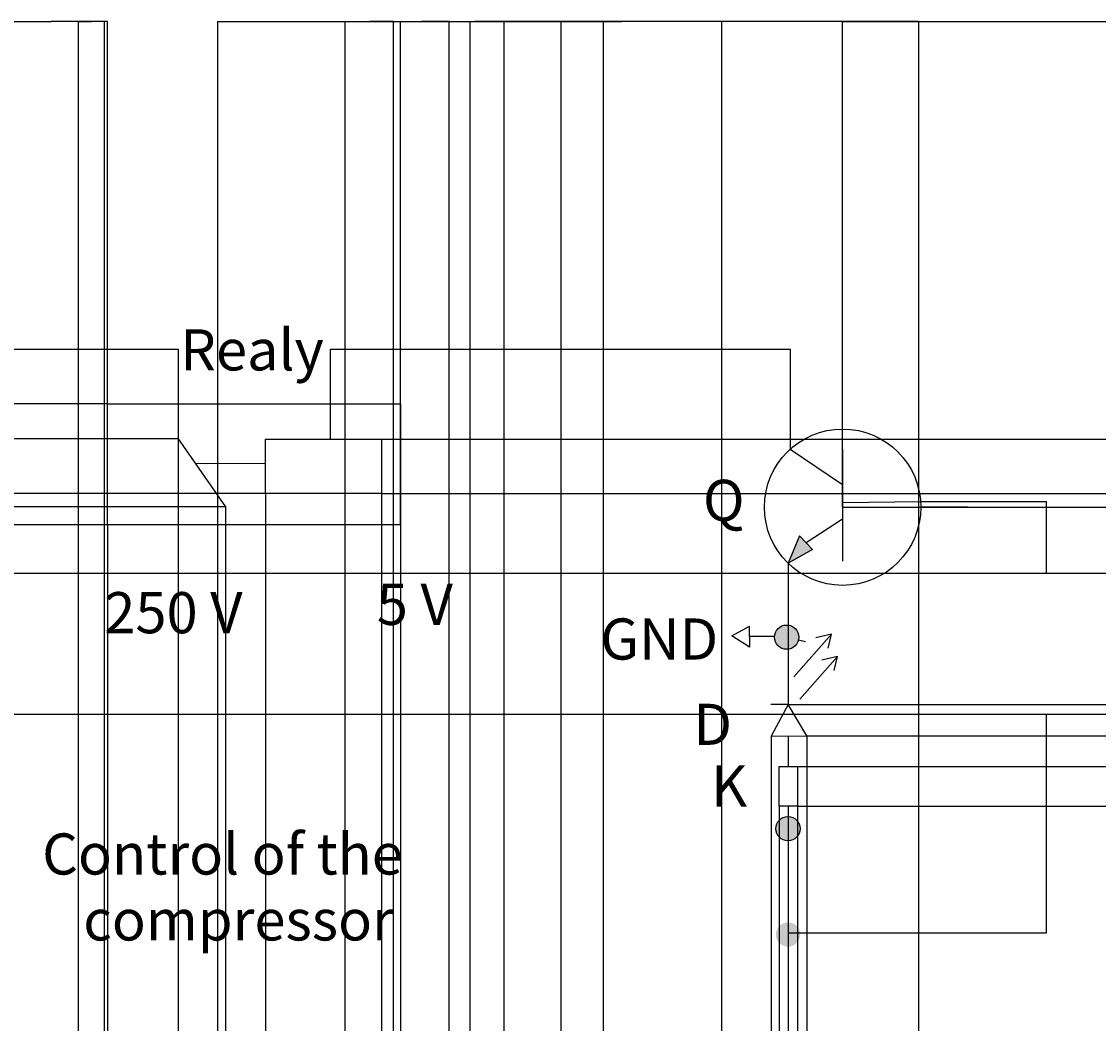
# Model space of a CAD drawing. Units: inches. Extents: x 35362 to 73946, y 43607 to 67532.
# Tile 132 of 134: x 52056 to 57838, y 62152 to 67532. Entities that reach past the tile are written whole.
import ezdxf

# ---------------------------------------------------------------- set-up
doc = ezdxf.new("R2010")
doc.units = ezdxf.units.IN
doc.header["$MEASUREMENT"] = 0
for name, color, linetype, lineweight in [('A-ANNO-DIMS', 2, 'Continuous', 18), ('E-ANNO-TEXT', 5, 'Continuous', 18), ('E-SYMB', 1, 'Continuous', 25), ('E-SYMB-PATT', 1, 'Continuous', 13), ('E-WIRE', 3, 'Continuous', 25)]:
    doc.layers.add(name, color=color, linetype=linetype, lineweight=lineweight)
doc.styles.get("Standard").update_dxf_attribs({"font": 'arial.ttf'})
doc.dimstyles.get("Standard").update_dxf_attribs({"dimtxt": 0.18, "dimasz": 0.18, "dimexe": 0.18, "dimexo": 0.0625, "dimgap": 0.09, "dimtad": 0, "dimtih": 1, "dimtoh": 1, "dimdec": 4, "dimzin": 0, "dimdsep": 46, "dimtxsty": 'Standard', "dimcen": 0.09, "dimadec": 0, "dimazin": 0, "dimtfac": 1, "dimtdec": 4, "dimtofl": 0, "dimtmove": 0, "dimatfit": 3, "dimfxl": 1, "dimtolj": 1, "dimtzin": 0, "dimarcsym": 0})

# ---------------------------------------------------------------- blocks, each defined once
blk = doc.blocks.new('*D9')
at = {"layer": 'A-ANNO-DIMS', "color": 0, "lineweight": -2, "transparency": 16777216}
for p, q in [((56873.6, 59185.2), (56873.6, 67531.7)), ((56873.8, 67531.5), (59056.9, 67531.5)), ((61240.7, 67531.5), (59057.6, 67531.5)), ((61240.9, 59185.2), (61240.9, 67531.7))]:
    blk.add_line(p, q, dxfattribs=at)
at = {"layer": 'A-ANNO-DIMS', "color": 0, "transparency": 16777216}
for points in [[(56873.8, 67531.5), (56873.8, 67531.5), (56873.6, 67531.5)], [(61240.7, 67531.5), (61240.7, 67531.5), (61240.9, 67531.5)]]:
    blk.add_solid(points, dxfattribs=at)
at = {"layer": 'Defpoints', "color": 0, "transparency": 16777216}
for p in [(61240.9, 67531.5), (56873.6, 59185.1), (61240.9, 59185.1)]:
    blk.add_point(p, dxfattribs=at)
at = {"layer": 'A-ANNO-DIMS', "color": 0, "transparency": 16777216, "insert": (59057.3, 67531.5), "char_height": 0.18, "attachment_point": 5}
blk.add_mtext('\\A1;4367', dxfattribs=at)
blk = doc.blocks.new('*D20')
at = {"layer": 'A-ANNO-DIMS', "color": 0, "lineweight": -2, "transparency": 16777216}
for p, q in [((56464.6, 64923.8), (56464.8, 64923.8)), ((56464.7, 64923.7), (56464.7, 64923.8)), ((57136.4, 64924), (56884.7, 64923.9))]:
    blk.add_line(p, q, dxfattribs=at)
at = {"layer": 'A-ANNO-DIMS', "color": 0, "transparency": 16777216}
blk.add_solid([(56884.7, 64923.9), (56884.7, 64923.8), (56884.5, 64923.9)], dxfattribs=at)
at = {"layer": 'Defpoints', "color": 0, "transparency": 16777216}
for p in [(56044.9, 64923.6), (56884.5, 64923.9)]:
    blk.add_point(p, dxfattribs=at)
at = {"layer": 'A-ANNO-DIMS', "color": 0, "transparency": 16777216, "insert": (57137.1, 64924), "char_height": 0.18, "attachment_point": 5}
blk.add_mtext('\\A1;2X ∅839.6', dxfattribs=at)
blk = doc.blocks.new('*D22')
at = {"layer": 'A-ANNO-DIMS', "color": 0, "lineweight": -2, "transparency": 16777216}
for p, q in [((56163.8, 64225.8), (56164, 64225.8)), ((56163.9, 64225.7), (56163.9, 64225.9)), ((56265.4, 64201.7), (56227.5, 64210.7))]:
    blk.add_line(p, q, dxfattribs=at)
at = {"layer": 'A-ANNO-DIMS', "color": 0, "transparency": 16777216}
blk.add_solid([(56227.5, 64210.7), (56227.5, 64210.7), (56227.3, 64210.7)], dxfattribs=at)
at = {"layer": 'Defpoints', "color": 0, "transparency": 16777216}
for p in [(56100.5, 64240.9), (56227.3, 64210.7)]:
    blk.add_point(p, dxfattribs=at)
at = {"layer": 'A-ANNO-DIMS', "color": 0, "transparency": 16777216, "insert": (56266.1, 64201.7), "char_height": 0.18, "attachment_point": 5}
blk.add_mtext('\\A1;4X ∅130.4', dxfattribs=at)
blk = doc.blocks.new('*D25')
at = {"layer": 'A-ANNO-DIMS', "color": 0, "lineweight": -2, "transparency": 16777216}
for p, q in [((53109.8, 59023.3), (53109.8, 67531.7)), ((53109.9, 67531.5), (54991.2, 67531.5)), ((56873.4, 67531.5), (54992.1, 67531.5)), ((56873.6, 59185.2), (56873.6, 67531.7))]:
    blk.add_line(p, q, dxfattribs=at)
at = {"layer": 'A-ANNO-DIMS', "color": 0, "transparency": 16777216}
for points in [[(53109.9, 67531.5), (53109.9, 67531.5), (53109.8, 67531.5)], [(56873.4, 67531.5), (56873.4, 67531.5), (56873.6, 67531.5)]]:
    blk.add_solid(points, dxfattribs=at)
at = {"layer": 'Defpoints', "color": 0, "transparency": 16777216}
for p in [(56873.6, 67531.5), (56873.6, 59185.1), (53109.8, 59023.3)]:
    blk.add_point(p, dxfattribs=at)
at = {"layer": 'A-ANNO-DIMS', "color": 0, "transparency": 16777216, "insert": (54991.7, 67531.5), "char_height": 0.18, "attachment_point": 5}
blk.add_mtext('\\A1;3763.8', dxfattribs=at)
blk = doc.blocks.new('*D29')
at = {"layer": 'A-ANNO-DIMS', "color": 0, "lineweight": -2, "transparency": 16777216}
for p, q in [((51913.9, 64127.5), (51913.9, 67531.7)), ((51914.1, 67531.5), (52215.5, 67531.5)), ((52517.6, 67531.5), (52216.3, 67531.5)), ((52517.8, 64828.6), (52517.8, 67531.7))]:
    blk.add_line(p, q, dxfattribs=at)
at = {"layer": 'A-ANNO-DIMS', "color": 0, "transparency": 16777216}
for points in [[(51914.1, 67531.5), (51914.1, 67531.5), (51913.9, 67531.5)], [(52517.6, 67531.5), (52517.6, 67531.5), (52517.8, 67531.5)]]:
    blk.add_solid(points, dxfattribs=at)
at = {"layer": 'Defpoints', "color": 0, "transparency": 16777216}
for p in [(52517.8, 67531.5), (52517.8, 64828.6), (51913.9, 64127.4)]:
    blk.add_point(p, dxfattribs=at)
at = {"layer": 'A-ANNO-DIMS', "color": 0, "transparency": 16777216, "insert": (52215.9, 67531.5), "char_height": 0.18, "attachment_point": 5}
blk.add_mtext('\\A1;603.9', dxfattribs=at)
blk = doc.blocks.new('*D30')
at = {"layer": 'A-ANNO-DIMS', "color": 0, "lineweight": -2, "transparency": 16777216}
for p, q in [((54090.8, 64828.6), (54090.8, 67531.7)), ((54090.9, 67531.5), (55277.3, 67531.5)), ((56464.6, 67531.5), (55278.2, 67531.5)), ((56464.7, 64923.8), (56464.7, 67531.7))]:
    blk.add_line(p, q, dxfattribs=at)
at = {"layer": 'A-ANNO-DIMS', "color": 0, "transparency": 16777216}
for points in [[(54090.9, 67531.5), (54090.9, 67531.5), (54090.8, 67531.5)], [(56464.6, 67531.5), (56464.6, 67531.5), (56464.7, 67531.5)]]:
    blk.add_solid(points, dxfattribs=at)
at = {"layer": 'Defpoints', "color": 0, "transparency": 16777216}
for p in [(56464.7, 67531.5), (56464.7, 64923.8), (54090.8, 64828.6)]:
    blk.add_point(p, dxfattribs=at)
at = {"layer": 'A-ANNO-DIMS', "color": 0, "transparency": 16777216, "insert": (55277.8, 67531.5), "char_height": 0.18, "attachment_point": 5}
blk.add_mtext('\\A1;2374.0', dxfattribs=at)
blk = doc.blocks.new('*D31')
at = {"layer": 'A-ANNO-DIMS', "color": 0, "lineweight": -2, "transparency": 16777216}
for p, q in [((56464.7, 64923.8), (56464.7, 67531.7)), ((56464.9, 67531.5), (58624.5, 67531.5)), ((60785, 67531.5), (58625.4, 67531.5)), ((60785.2, 64923.8), (60785.2, 67531.7))]:
    blk.add_line(p, q, dxfattribs=at)
at = {"layer": 'A-ANNO-DIMS', "color": 0, "transparency": 16777216}
for points in [[(56464.9, 67531.5), (56464.9, 67531.5), (56464.7, 67531.5)], [(60785, 67531.5), (60785, 67531.5), (60785.2, 67531.5)]]:
    blk.add_solid(points, dxfattribs=at)
at = {"layer": 'Defpoints', "color": 0, "transparency": 16777216}
for p in [(60785.2, 67531.5), (56464.7, 64923.8), (60785.2, 64923.8)]:
    blk.add_point(p, dxfattribs=at)
at = {"layer": 'A-ANNO-DIMS', "color": 0, "transparency": 16777216, "insert": (58625, 67531.5), "char_height": 0.18, "attachment_point": 5}
blk.add_mtext('\\A1;4320.5', dxfattribs=at)
blk = doc.blocks.new('*D39')
at = {"layer": 'A-ANNO-DIMS', "color": 0, "lineweight": -2, "transparency": 16777216}
for p, q in [((53793.6, 46128.9), (53793.6, 67531.7)), ((53793.8, 67531.5), (54487.2, 67531.5)), ((55181.5, 67531.5), (54488.1, 67531.5)), ((55181.6, 46128.9), (55181.6, 67531.7))]:
    blk.add_line(p, q, dxfattribs=at)
at = {"layer": 'A-ANNO-DIMS', "color": 0, "transparency": 16777216}
for points in [[(53793.8, 67531.5), (53793.8, 67531.5), (53793.6, 67531.5)], [(55181.5, 67531.5), (55181.5, 67531.5), (55181.6, 67531.5)]]:
    blk.add_solid(points, dxfattribs=at)
at = {"layer": 'Defpoints', "color": 0, "transparency": 16777216}
for p in [(55181.6, 67531.5), (53793.6, 46128.9), (55181.6, 46128.9)]:
    blk.add_point(p, dxfattribs=at)
at = {"layer": 'A-ANNO-DIMS', "color": 0, "transparency": 16777216, "insert": (54487.6, 67531.5), "char_height": 0.18, "attachment_point": 5}
blk.add_mtext('\\A1;1388.0', dxfattribs=at)
blk = doc.blocks.new('*D44')
at = {"layer": 'A-ANNO-DIMS', "color": 0, "lineweight": -2, "transparency": 16777216}
for p, q in [((52517.8, 64828.5), (52517.8, 43606.7)), ((54090.8, 64828.5), (54090.8, 43606.7)), ((52518, 43606.9), (53303.8, 43606.9)), ((54090.6, 43606.9), (53304.7, 43606.9))]:
    blk.add_line(p, q, dxfattribs=at)
at = {"layer": 'A-ANNO-DIMS', "color": 0, "transparency": 16777216}
for points in [[(52518, 43606.9), (52518, 43606.8), (52517.8, 43606.9)], [(54090.6, 43606.9), (54090.6, 43606.8), (54090.8, 43606.9)]]:
    blk.add_solid(points, dxfattribs=at)
at = {"layer": 'Defpoints', "color": 0, "transparency": 16777216}
for p in [(52517.8, 64828.6), (54090.8, 64828.6), (54090.8, 43606.9)]:
    blk.add_point(p, dxfattribs=at)
at = {"layer": 'A-ANNO-DIMS', "color": 0, "transparency": 16777216, "insert": (53304.3, 43606.9), "char_height": 0.18, "attachment_point": 5}
blk.add_mtext('\\A1;1573.0', dxfattribs=at)
blk = doc.blocks.new('*D45')
at = {"layer": 'A-ANNO-DIMS', "color": 0, "lineweight": -2, "transparency": 16777216}
for p, q in [((52517.7, 65478.9), (35361.8, 65478.9)), ((35361.9, 65478.7), (35361.9, 65153.9)), ((35361.9, 64828.7), (35361.9, 65153.5)), ((52517.7, 64828.6), (35361.8, 64828.6))]:
    blk.add_line(p, q, dxfattribs=at)
at = {"layer": 'A-ANNO-DIMS', "color": 0, "transparency": 16777216}
for points in [[(35361.9, 65478.7), (35362, 65478.7), (35361.9, 65478.9)], [(35361.9, 64828.7), (35362, 64828.7), (35361.9, 64828.6)]]:
    blk.add_solid(points, dxfattribs=at)
at = {"layer": 'Defpoints', "color": 0, "transparency": 16777216}
for p in [(52517.8, 65478.9), (35361.9, 64828.6), (52517.8, 64828.6)]:
    blk.add_point(p, dxfattribs=at)
at = {"layer": 'A-ANNO-DIMS', "color": 0, "transparency": 16777216, "insert": (35361.9, 65153.7), "char_height": 0.18, "attachment_point": 5}
blk.add_mtext('\\A1;650.3', dxfattribs=at)
blk = doc.blocks.new('*D51')
at = {"layer": 'A-ANNO-DIMS', "color": 0, "lineweight": -2, "transparency": 16777216}
for p, q in [((56873.6, 59185.2), (56873.6, 67531.7)), ((56873.8, 67531.5), (57886, 67531.5)), ((58899.2, 67531.5), (57887, 67531.5)), ((58899.4, 59601.5), (58899.4, 67531.7))]:
    blk.add_line(p, q, dxfattribs=at)
at = {"layer": 'A-ANNO-DIMS', "color": 0, "transparency": 16777216}
for points in [[(56873.8, 67531.5), (56873.8, 67531.5), (56873.6, 67531.5)], [(58899.2, 67531.5), (58899.2, 67531.5), (58899.4, 67531.5)]]:
    blk.add_solid(points, dxfattribs=at)
at = {"layer": 'Defpoints', "color": 0, "transparency": 16777216}
for p in [(58899.4, 67531.5), (58899.4, 59601.5), (56873.6, 59185.1)]:
    blk.add_point(p, dxfattribs=at)
at = {"layer": 'A-ANNO-DIMS', "color": 0, "transparency": 16777216, "insert": (57886.5, 67531.5), "char_height": 0.18, "attachment_point": 5}
blk.add_mtext('\\A1;2025.8', dxfattribs=at)
blk = doc.blocks.new('*D60')
at = {"layer": 'A-ANNO-DIMS', "color": 0, "lineweight": -2, "transparency": 16777216}
for p, q in [((56464.6, 64923.8), (56464.8, 64923.8)), ((56464.7, 64923.7), (56464.7, 64923.8)), ((57136.4, 64924), (56884.7, 64923.9))]:
    blk.add_line(p, q, dxfattribs=at)
at = {"layer": 'A-ANNO-DIMS', "color": 0, "transparency": 16777216}
blk.add_solid([(56884.7, 64923.9), (56884.7, 64923.8), (56884.5, 64923.9)], dxfattribs=at)
at = {"layer": 'Defpoints', "color": 0, "transparency": 16777216}
for p in [(56044.9, 64923.6), (56884.5, 64923.9)]:
    blk.add_point(p, dxfattribs=at)
at = {"layer": 'A-ANNO-DIMS', "color": 0, "transparency": 16777216, "insert": (57137.1, 64924), "char_height": 0.18, "attachment_point": 5}
blk.add_mtext('\\A1;2X ∅839.6', dxfattribs=at)
blk = doc.blocks.new('*D62')
at = {"layer": 'A-ANNO-DIMS', "color": 0, "lineweight": -2, "transparency": 16777216}
for p, q in [((56163.8, 64225.8), (56164, 64225.8)), ((56163.9, 64225.7), (56163.9, 64225.9)), ((56265.4, 64201.7), (56227.5, 64210.7))]:
    blk.add_line(p, q, dxfattribs=at)
at = {"layer": 'A-ANNO-DIMS', "color": 0, "transparency": 16777216}
blk.add_solid([(56227.5, 64210.7), (56227.5, 64210.7), (56227.3, 64210.7)], dxfattribs=at)
at = {"layer": 'Defpoints', "color": 0, "transparency": 16777216}
for p in [(56100.5, 64240.9), (56227.3, 64210.7)]:
    blk.add_point(p, dxfattribs=at)
at = {"layer": 'A-ANNO-DIMS', "color": 0, "transparency": 16777216, "insert": (56266.1, 64201.7), "char_height": 0.18, "attachment_point": 5}
blk.add_mtext('\\A1;4X ∅130.4', dxfattribs=at)
blk = doc.blocks.new('*D73')
at = {"layer": 'A-ANNO-DIMS', "color": 0, "lineweight": -2, "transparency": 16777216}
for p, q in [((59468.7, 64568), (35361.8, 64568)), ((35361.9, 64567.8), (35361.9, 64189.8)), ((35361.9, 63811.5), (35361.9, 64189.5)), ((59468.7, 63811.4), (35361.8, 63811.4))]:
    blk.add_line(p, q, dxfattribs=at)
at = {"layer": 'A-ANNO-DIMS', "color": 0, "transparency": 16777216}
for points in [[(35361.9, 64567.8), (35362, 64567.8), (35361.9, 64568)], [(35361.9, 63811.5), (35362, 63811.5), (35361.9, 63811.4)]]:
    blk.add_solid(points, dxfattribs=at)
at = {"layer": 'Defpoints', "color": 0, "transparency": 16777216}
for p in [(35361.9, 64568), (59468.8, 64568), (59468.8, 63811.4)]:
    blk.add_point(p, dxfattribs=at)
at = {"layer": 'A-ANNO-DIMS', "color": 0, "transparency": 16777216, "insert": (35361.9, 64189.7), "char_height": 0.18, "attachment_point": 5}
blk.add_mtext('\\A1;756.6', dxfattribs=at)
blk = doc.blocks.new('*D77')
at = {"layer": 'A-ANNO-DIMS', "color": 0, "lineweight": -2, "transparency": 16777216}
for p, q in [((53793.6, 46128.9), (53793.6, 67531.7)), ((53793.8, 67531.5), (53922.8, 67531.5)), ((54052.7, 67531.5), (53923.7, 67531.5)), ((54052.9, 46555.4), (54052.9, 67531.7))]:
    blk.add_line(p, q, dxfattribs=at)
at = {"layer": 'A-ANNO-DIMS', "color": 0, "transparency": 16777216}
for points in [[(53793.8, 67531.5), (53793.8, 67531.5), (53793.6, 67531.5)], [(54052.7, 67531.5), (54052.7, 67531.5), (54052.9, 67531.5)]]:
    blk.add_solid(points, dxfattribs=at)
at = {"layer": 'Defpoints', "color": 0, "transparency": 16777216}
for p in [(54052.9, 67531.5), (54052.9, 46555.3), (53793.6, 46128.9)]:
    blk.add_point(p, dxfattribs=at)
at = {"layer": 'A-ANNO-DIMS', "color": 0, "transparency": 16777216, "insert": (53923.3, 67531.5), "char_height": 0.18, "attachment_point": 5}
blk.add_mtext('\\A1;259.26', dxfattribs=at)
blk = doc.blocks.new('*D78')
at = {"layer": 'A-ANNO-DIMS', "color": 0, "lineweight": -2, "transparency": 16777216}
for p, q in [((54052.9, 46555.4), (54052.9, 67531.7)), ((54053.1, 67531.5), (54202.6, 67531.5)), ((54352.9, 67531.5), (54203.4, 67531.5)), ((54353.1, 46555.4), (54353.1, 67531.7))]:
    blk.add_line(p, q, dxfattribs=at)
at = {"layer": 'A-ANNO-DIMS', "color": 0, "transparency": 16777216}
for points in [[(54053.1, 67531.5), (54053.1, 67531.5), (54052.9, 67531.5)], [(54352.9, 67531.5), (54352.9, 67531.5), (54353.1, 67531.5)]]:
    blk.add_solid(points, dxfattribs=at)
at = {"layer": 'Defpoints', "color": 0, "transparency": 16777216}
for p in [(54353.1, 67531.5), (54052.9, 46555.3), (54353.1, 46555.3)]:
    blk.add_point(p, dxfattribs=at)
at = {"layer": 'A-ANNO-DIMS', "color": 0, "transparency": 16777216, "insert": (54203, 67531.5), "char_height": 0.18, "attachment_point": 5}
blk.add_mtext('\\A1;300.2', dxfattribs=at)
blk = doc.blocks.new('*D79')
at = {"layer": 'A-ANNO-DIMS', "color": 0, "lineweight": -2, "transparency": 16777216}
for p, q in [((54353.1, 46555.4), (54353.1, 67531.7)), ((54353.3, 67531.5), (54500.2, 67531.5)), ((54648, 67531.5), (54501, 67531.5)), ((54648.2, 46555.4), (54648.2, 67531.7))]:
    blk.add_line(p, q, dxfattribs=at)
at = {"layer": 'A-ANNO-DIMS', "color": 0, "transparency": 16777216}
for points in [[(54353.3, 67531.5), (54353.3, 67531.5), (54353.1, 67531.5)], [(54648, 67531.5), (54648, 67531.5), (54648.2, 67531.5)]]:
    blk.add_solid(points, dxfattribs=at)
at = {"layer": 'Defpoints', "color": 0, "transparency": 16777216}
for p in [(54648.2, 67531.5), (54353.1, 46555.3), (54648.2, 46555.3)]:
    blk.add_point(p, dxfattribs=at)
at = {"layer": 'A-ANNO-DIMS', "color": 0, "transparency": 16777216, "insert": (54500.6, 67531.5), "char_height": 0.18, "attachment_point": 5}
blk.add_mtext('\\A1;295.1', dxfattribs=at)
blk = doc.blocks.new('*D80')
at = {"layer": 'A-ANNO-DIMS', "color": 0, "lineweight": -2, "transparency": 16777216}
for p, q in [((54648.2, 46555.4), (54648.2, 67531.7)), ((54648.4, 67531.5), (54800.3, 67531.5)), ((54953.3, 67531.5), (54801.3, 67531.5)), ((54953.4, 46555.4), (54953.4, 67531.7))]:
    blk.add_line(p, q, dxfattribs=at)
at = {"layer": 'A-ANNO-DIMS', "color": 0, "transparency": 16777216}
for points in [[(54648.4, 67531.5), (54648.4, 67531.5), (54648.2, 67531.5)], [(54953.3, 67531.5), (54953.3, 67531.5), (54953.4, 67531.5)]]:
    blk.add_solid(points, dxfattribs=at)
at = {"layer": 'Defpoints', "color": 0, "transparency": 16777216}
for p in [(54953.4, 67531.5), (54648.2, 46555.3), (54953.4, 46555.3)]:
    blk.add_point(p, dxfattribs=at)
at = {"layer": 'A-ANNO-DIMS', "color": 0, "transparency": 16777216, "insert": (54800.8, 67531.5), "char_height": 0.18, "attachment_point": 5}
blk.add_mtext('\\A1;305.27', dxfattribs=at)
blk = doc.blocks.new('*D82')
at = {"layer": 'A-ANNO-DIMS', "color": 0, "lineweight": -2, "transparency": 16777216}
for p, q in [((54464.4, 49314.7), (54464.4, 67531.7)), ((54464.6, 67531.5), (55139.4, 67531.5)), ((55815.1, 67531.5), (55140.3, 67531.5)), ((55815.3, 49110.2), (55815.3, 67531.7))]:
    blk.add_line(p, q, dxfattribs=at)
at = {"layer": 'A-ANNO-DIMS', "color": 0, "transparency": 16777216}
for points in [[(54464.6, 67531.5), (54464.6, 67531.5), (54464.4, 67531.5)], [(55815.1, 67531.5), (55815.1, 67531.5), (55815.3, 67531.5)]]:
    blk.add_solid(points, dxfattribs=at)
at = {"layer": 'Defpoints', "color": 0, "transparency": 16777216}
for p in [(55815.3, 67531.5), (54464.4, 49314.7), (55815.3, 49110.1)]:
    blk.add_point(p, dxfattribs=at)
at = {"layer": 'A-ANNO-DIMS', "color": 0, "transparency": 16777216, "insert": (55139.9, 67531.5), "char_height": 0.18, "attachment_point": 5}
blk.add_mtext('\\A1;1350.9', dxfattribs=at)
blk = doc.blocks.new('*D88')
at = {"layer": 'A-ANNO-DIMS', "color": 0, "lineweight": -2, "transparency": 16777216}
for p, q in [((52362.6, 48318.3), (52362.6, 67531.7)), ((52362.7, 67531.5), (52432.1, 67531.5)), ((52502.2, 67531.5), (52432.8, 67531.5)), ((52502.4, 48318.3), (52502.4, 67531.7))]:
    blk.add_line(p, q, dxfattribs=at)
at = {"layer": 'A-ANNO-DIMS', "color": 0, "transparency": 16777216}
for points in [[(52362.7, 67531.5), (52362.7, 67531.5), (52362.6, 67531.5)], [(52502.2, 67531.5), (52502.2, 67531.5), (52502.4, 67531.5)]]:
    blk.add_solid(points, dxfattribs=at)
at = {"layer": 'Defpoints', "color": 0, "transparency": 16777216}
for p in [(52502.4, 67531.5), (52362.6, 48318.3), (52502.4, 48318.3)]:
    blk.add_point(p, dxfattribs=at)
at = {"layer": 'A-ANNO-DIMS', "color": 0, "transparency": 16777216, "insert": (52432.5, 67531.5), "char_height": 0.18, "attachment_point": 5}
blk.add_mtext('\\A1;139.8', dxfattribs=at)
blk = doc.blocks.new('*D96')
at = {"layer": 'A-ANNO-DIMS', "color": 0, "lineweight": -2, "transparency": 16777216}
for p, q in [((53366.8, 64997.6), (53366.8, 43606.7)), ((53988.6, 64997.6), (53988.6, 43606.7)), ((53366.9, 43606.9), (53677.3, 43606.9)), ((53988.4, 43606.9), (53678.1, 43606.9))]:
    blk.add_line(p, q, dxfattribs=at)
at = {"layer": 'A-ANNO-DIMS', "color": 0, "transparency": 16777216}
for points in [[(53366.9, 43606.9), (53366.9, 43606.8), (53366.8, 43606.9)], [(53988.4, 43606.9), (53988.4, 43606.8), (53988.6, 43606.9)]]:
    blk.add_solid(points, dxfattribs=at)
at = {"layer": 'Defpoints', "color": 0, "transparency": 16777216}
for p in [(53366.8, 64997.7), (53988.6, 64997.7), (53988.6, 43606.9)]:
    blk.add_point(p, dxfattribs=at)
at = {"layer": 'A-ANNO-DIMS', "color": 0, "transparency": 16777216, "insert": (53677.7, 43606.9), "char_height": 0.18, "attachment_point": 5}
blk.add_mtext('\\A1;621.8', dxfattribs=at)
blk = doc.blocks.new('*D97')
at = {"layer": 'A-ANNO-DIMS', "color": 0, "lineweight": -2, "transparency": 16777216}
for p, q in [((53988.7, 65288.9), (73945.8, 65288.9)), ((73945.6, 65288.7), (73945.6, 65143.5)), ((73945.6, 64997.9), (73945.6, 65143.1)), ((53988.7, 64997.7), (73945.8, 64997.7))]:
    blk.add_line(p, q, dxfattribs=at)
at = {"layer": 'A-ANNO-DIMS', "color": 0, "transparency": 16777216}
for points in [[(73945.6, 65288.7), (73945.7, 65288.7), (73945.6, 65288.9)], [(73945.6, 64997.9), (73945.7, 64997.9), (73945.6, 64997.7)]]:
    blk.add_solid(points, dxfattribs=at)
at = {"layer": 'Defpoints', "color": 0, "transparency": 16777216}
for p in [(53988.6, 65288.9), (73945.6, 65288.9), (53988.6, 64997.7)]:
    blk.add_point(p, dxfattribs=at)
at = {"layer": 'A-ANNO-DIMS', "color": 0, "transparency": 16777216, "insert": (73945.6, 65143.3), "char_height": 0.18, "attachment_point": 5}
blk.add_mtext('\\A1;291.2', dxfattribs=at)
blk = doc.blocks.new('*D98')
at = {"layer": 'A-ANNO-DIMS', "color": 0, "lineweight": -2, "transparency": 16777216}
for p, q in [((53366.7, 64997.7), (35361.8, 64997.7)), ((35361.9, 64997.5), (35361.9, 64913.3)), ((35361.9, 64828.7), (35361.9, 64912.9)), ((52517.7, 64828.6), (35361.8, 64828.6))]:
    blk.add_line(p, q, dxfattribs=at)
at = {"layer": 'A-ANNO-DIMS', "color": 0, "transparency": 16777216}
for points in [[(35361.9, 64997.5), (35362, 64997.5), (35361.9, 64997.7)], [(35361.9, 64828.7), (35362, 64828.7), (35361.9, 64828.6)]]:
    blk.add_solid(points, dxfattribs=at)
at = {"layer": 'Defpoints', "color": 0, "transparency": 16777216}
for p in [(53366.8, 64997.7), (35361.9, 64828.6), (52517.8, 64828.6)]:
    blk.add_point(p, dxfattribs=at)
at = {"layer": 'A-ANNO-DIMS', "color": 0, "transparency": 16777216, "insert": (35361.9, 64913.1), "char_height": 0.18, "attachment_point": 5}
blk.add_mtext('\\A1;169.13', dxfattribs=at)
blk = doc.blocks.new('*D99')
at = {"layer": 'A-ANNO-DIMS', "color": 0, "lineweight": -2, "transparency": 16777216}
for p, q in [((52897.5, 65291.5), (52897.5, 43606.7)), ((52517.8, 64828.5), (52517.8, 43606.7)), ((52518, 43606.9), (52707.2, 43606.9)), ((52897.3, 43606.9), (52708, 43606.9))]:
    blk.add_line(p, q, dxfattribs=at)
at = {"layer": 'A-ANNO-DIMS', "color": 0, "transparency": 16777216}
for points in [[(52518, 43606.9), (52518, 43606.8), (52517.8, 43606.9)], [(52897.3, 43606.9), (52897.3, 43606.8), (52897.5, 43606.9)]]:
    blk.add_solid(points, dxfattribs=at)
at = {"layer": 'Defpoints', "color": 0, "transparency": 16777216}
for p in [(52897.5, 65291.6), (52517.8, 64828.6), (52897.5, 43606.9)]:
    blk.add_point(p, dxfattribs=at)
at = {"layer": 'A-ANNO-DIMS', "color": 0, "transparency": 16777216, "insert": (52707.6, 43606.9), "char_height": 0.18, "attachment_point": 5}
blk.add_mtext('\\A1;379.7', dxfattribs=at)
blk = doc.blocks.new('*D100')
at = {"layer": 'A-ANNO-DIMS', "color": 0, "lineweight": -2, "transparency": 16777216}
for p, q in [((52897.5, 65291.5), (52897.5, 43606.7)), ((53150.7, 64926.1), (53150.7, 43606.7)), ((52897.7, 43606.9), (53023.7, 43606.9)), ((53150.5, 43606.9), (53024.5, 43606.9))]:
    blk.add_line(p, q, dxfattribs=at)
at = {"layer": 'A-ANNO-DIMS', "color": 0, "transparency": 16777216}
for points in [[(52897.7, 43606.9), (52897.7, 43606.8), (52897.5, 43606.9)], [(53150.5, 43606.9), (53150.5, 43606.8), (53150.7, 43606.9)]]:
    blk.add_solid(points, dxfattribs=at)
at = {"layer": 'Defpoints', "color": 0, "transparency": 16777216}
for p in [(52897.5, 65291.6), (53150.7, 64926.1), (53150.7, 43606.9)]:
    blk.add_point(p, dxfattribs=at)
at = {"layer": 'A-ANNO-DIMS', "color": 0, "transparency": 16777216, "insert": (53024.1, 43606.9), "char_height": 0.18, "attachment_point": 5}
blk.add_mtext('\\A1;253.2', dxfattribs=at)
blk = doc.blocks.new('*D101')
at = {"layer": 'A-ANNO-DIMS', "color": 0, "lineweight": -2, "transparency": 16777216}
for p, q in [((52897.4, 65291.6), (35361.8, 65291.6)), ((35361.9, 65291.4), (35361.9, 65109)), ((35361.9, 64926.3), (35361.9, 65108.7)), ((53150.6, 64926.1), (35361.8, 64926.1))]:
    blk.add_line(p, q, dxfattribs=at)
at = {"layer": 'A-ANNO-DIMS', "color": 0, "transparency": 16777216}
for points in [[(35361.9, 65291.4), (35362, 65291.4), (35361.9, 65291.6)], [(35361.9, 64926.3), (35362, 64926.3), (35361.9, 64926.1)]]:
    blk.add_solid(points, dxfattribs=at)
at = {"layer": 'Defpoints', "color": 0, "transparency": 16777216}
for p in [(52897.5, 65291.6), (35361.9, 64926.1), (53150.7, 64926.1)]:
    blk.add_point(p, dxfattribs=at)
at = {"layer": 'A-ANNO-DIMS', "color": 0, "transparency": 16777216, "insert": (35361.9, 65108.9), "char_height": 0.18, "attachment_point": 5}
blk.add_mtext('\\A1;365.45', dxfattribs=at)
blk = doc.blocks.new('*D102')
at = {"layer": 'A-ANNO-DIMS', "color": 0, "lineweight": -2, "transparency": 16777216}
for p, q in [((56080.5, 63694.7), (56080.5, 43606.7)), ((56272.5, 63696.8), (56272.5, 43606.7)), ((56080.7, 43606.9), (56176, 43606.9)), ((56272.3, 43606.9), (56176.9, 43606.9))]:
    blk.add_line(p, q, dxfattribs=at)
at = {"layer": 'A-ANNO-DIMS', "color": 0, "transparency": 16777216}
for points in [[(56080.7, 43606.9), (56080.7, 43606.8), (56080.5, 43606.9)], [(56272.3, 43606.9), (56272.3, 43606.8), (56272.5, 43606.9)]]:
    blk.add_solid(points, dxfattribs=at)
at = {"layer": 'Defpoints', "color": 0, "transparency": 16777216}
for p in [(56080.5, 63694.8), (56272.5, 63696.9), (56272.5, 43606.9)]:
    blk.add_point(p, dxfattribs=at)
at = {"layer": 'A-ANNO-DIMS', "color": 0, "transparency": 16777216, "insert": (56176.5, 43606.9), "char_height": 0.18, "attachment_point": 5}
blk.add_mtext('\\A1;191.98', dxfattribs=at)
blk = doc.blocks.new('*D103')
at = {"layer": 'A-ANNO-DIMS', "color": 0, "lineweight": -2, "transparency": 16777216}
for p, q in [((56172.1, 63863.5), (73945.8, 63863.5)), ((73945.6, 63863.3), (73945.6, 63780.4)), ((73945.6, 63697), (73945.6, 63780)), ((56272.5, 63696.9), (73945.8, 63696.9))]:
    blk.add_line(p, q, dxfattribs=at)
at = {"layer": 'A-ANNO-DIMS', "color": 0, "transparency": 16777216}
for points in [[(73945.6, 63863.3), (73945.7, 63863.3), (73945.6, 63863.5)], [(73945.6, 63697), (73945.7, 63697), (73945.6, 63696.9)]]:
    blk.add_solid(points, dxfattribs=at)
at = {"layer": 'Defpoints', "color": 0, "transparency": 16777216}
for p in [(56172.1, 63863.5), (73945.6, 63863.5), (56272.5, 63696.9)]:
    blk.add_point(p, dxfattribs=at)
at = {"layer": 'A-ANNO-DIMS', "color": 0, "transparency": 16777216, "insert": (73945.6, 63780.2), "char_height": 0.18, "attachment_point": 5}
blk.add_mtext('\\A1;166.62', dxfattribs=at)
blk = doc.blocks.new('*D104')
at = {"layer": 'A-ANNO-DIMS', "color": 0, "lineweight": -2, "transparency": 16777216}
for p, q in [((56123.2, 63318.1), (56123.2, 43606.7)), ((56223, 63318.1), (56223, 43606.7)), ((56123.4, 43606.9), (56172.7, 43606.9)), ((56222.8, 43606.9), (56173.5, 43606.9))]:
    blk.add_line(p, q, dxfattribs=at)
at = {"layer": 'A-ANNO-DIMS', "color": 0, "transparency": 16777216}
for points in [[(56123.4, 43606.9), (56123.4, 43606.8), (56123.2, 43606.9)], [(56222.8, 43606.9), (56222.8, 43606.8), (56223, 43606.9)]]:
    blk.add_solid(points, dxfattribs=at)
at = {"layer": 'Defpoints', "color": 0, "transparency": 16777216}
for p in [(56123.2, 63318.1), (56223, 63318.1), (56223, 43606.9)]:
    blk.add_point(p, dxfattribs=at)
at = {"layer": 'A-ANNO-DIMS', "color": 0, "transparency": 16777216, "insert": (56173.1, 43606.9), "char_height": 0.18, "attachment_point": 5}
blk.add_mtext('\\A1;99.74', dxfattribs=at)
blk = doc.blocks.new('*D105')
at = {"layer": 'A-ANNO-DIMS', "color": 0, "lineweight": -2, "transparency": 16777216}
for p, q in [((56223, 63531.5), (73945.8, 63531.5)), ((73945.6, 63531.3), (73945.6, 63425)), ((73945.6, 63318.3), (73945.6, 63424.6)), ((56223, 63318.1), (73945.8, 63318.1))]:
    blk.add_line(p, q, dxfattribs=at)
at = {"layer": 'A-ANNO-DIMS', "color": 0, "transparency": 16777216}
for points in [[(73945.6, 63531.3), (73945.7, 63531.3), (73945.6, 63531.5)], [(73945.6, 63318.3), (73945.7, 63318.3), (73945.6, 63318.1)]]:
    blk.add_solid(points, dxfattribs=at)
at = {"layer": 'Defpoints', "color": 0, "transparency": 16777216}
for p in [(56223, 63531.5), (73945.6, 63531.5), (56223, 63318.1)]:
    blk.add_point(p, dxfattribs=at)
at = {"layer": 'A-ANNO-DIMS', "color": 0, "transparency": 16777216, "insert": (73945.6, 63424.8), "char_height": 0.18, "attachment_point": 5}
blk.add_mtext('\\A1;213.36', dxfattribs=at)
blk = doc.blocks.new('*D106')
at = {"layer": 'A-ANNO-DIMS', "color": 0, "lineweight": -2, "transparency": 16777216}
for p, q in [((56464.8, 64923.8), (73945.8, 64923.8)), ((73945.6, 64923.6), (73945.6, 64393.8)), ((73945.6, 63863.7), (73945.6, 64393.4)), ((56172.1, 63863.5), (73945.8, 63863.5))]:
    blk.add_line(p, q, dxfattribs=at)
at = {"layer": 'A-ANNO-DIMS', "color": 0, "transparency": 16777216}
for points in [[(73945.6, 64923.6), (73945.7, 64923.6), (73945.6, 64923.8)], [(73945.6, 63863.7), (73945.7, 63863.7), (73945.6, 63863.5)]]:
    blk.add_solid(points, dxfattribs=at)
at = {"layer": 'Defpoints', "color": 0, "transparency": 16777216}
for p in [(56464.7, 64923.8), (56172.1, 63863.5), (73945.6, 63863.5)]:
    blk.add_point(p, dxfattribs=at)
at = {"layer": 'A-ANNO-DIMS', "color": 0, "transparency": 16777216, "insert": (73945.6, 64393.6), "char_height": 0.18, "attachment_point": 5}
blk.add_mtext('\\A1;1060.3', dxfattribs=at)
blk = doc.blocks.new('*D119')
at = {"layer": 'A-ANNO-DIMS', "color": 0, "lineweight": -2, "transparency": 16777216}
for p, q in [((56464.6, 64923.8), (56464.8, 64923.8)), ((56464.7, 64923.7), (56464.7, 64923.8)), ((57136.4, 64923.8), (56884.7, 64923.8))]:
    blk.add_line(p, q, dxfattribs=at)
at = {"layer": 'A-ANNO-DIMS', "color": 0, "transparency": 16777216}
blk.add_solid([(56884.7, 64923.8), (56884.7, 64923.7), (56884.5, 64923.8)], dxfattribs=at)
at = {"layer": 'Defpoints', "color": 0, "transparency": 16777216}
for p in [(56044.9, 64923.8), (56884.5, 64923.8)]:
    blk.add_point(p, dxfattribs=at)
at = {"layer": 'A-ANNO-DIMS', "color": 0, "transparency": 16777216, "insert": (57137.1, 64923.8), "char_height": 0.18, "attachment_point": 5}
blk.add_mtext('\\A1;2X ∅839.6', dxfattribs=at)

msp = doc.modelspace()

# ---------------------------------------------------------------- hatches: boundary and pattern name
at = {"layer": 'E-SYMB-PATT'}
h = msp.add_hatch(color=256, dxfattribs=at)
h.dxf.hatch_style = 1
h.paths.add_polyline_path([(56172.082, 64622.775), (56302.648, 64696.966), (56268.349, 64732.457), (56232.212, 64769.851)])
h = msp.add_hatch(color=256, dxfattribs=at)
h.dxf.hatch_style = 1
h.paths.add_polyline_path([(56163.909, 64291.021, 0.41421356), (56098.704, 64225.816, 0.41421356), (56163.909, 64160.611)])
h.paths.add_polyline_path([(56163.909, 64291.021), (56163.909, 64160.611, 0.41421356), (56229.114, 64225.816, 0.41421356)])
h = msp.add_hatch(color=256, dxfattribs=at)
h.dxf.hatch_style = 1
h.paths.add_polyline_path([(56171.65, 63262.799, 0.41421356), (56106.445, 63197.594, 0.41421356), (56171.65, 63132.389)])
h.paths.add_polyline_path([(56171.65, 63262.799), (56171.65, 63132.389, 0.41421356), (56236.855, 63197.594, 0.41421356)])
h = msp.add_hatch(color=256, dxfattribs=at)
h.dxf.hatch_style = 1
h.paths.add_polyline_path([(56171.65, 62694.154, 0.41421356), (56106.445, 62628.949, 0.41421356), (56171.65, 62563.744)])
h.paths.add_polyline_path([(56171.65, 62694.154), (56171.65, 62563.744, 0.41421356), (56236.855, 62628.949, 0.41421356)])

# ---------------------------------------------------------------- linework, layer by layer
at = {"layer": 'E-SYMB'}
for p, q in [((50978.723, 65771.512), (52897.48, 65771.512)), ((52897.48, 65771.512), (52897.48, 65446.355)), ((53715.699, 65432.662), (53715.699, 65771.512)), ((52897.48, 65446.355), (52897.48, 65291.589)), ((53715.699, 65288.889), (53715.699, 65432.662)), ((56183.372, 65390.542), (56183.372, 65234.625)), ((52897.48, 65291.589), (53150.662, 64926.138)), ((56183.372, 65234.625), (56464.734, 65045.794)), ((56464.734, 65234.625), (56464.734, 64749.552)), ((52988.698, 65159.922), (53366.766, 65159.117)), ((52897.48, 65011.857), (52897.48, 64533.201)), ((56883.598, 64951.784), (56464.734, 64947.861)), ((56464.734, 64859.406), (56268.349, 64732.457)), ((56232.212, 64769.851), (56172.082, 64622.775)), ((56268.349, 64732.457), (56232.212, 64769.851)), ((56302.648, 64696.966), (56172.082, 64622.775)), ((56268.349, 64732.457), (56302.648, 64696.966)), ((56464.734, 64749.552), (56464.734, 64633.387)), ((56172.082, 64622.775), (56172.082, 64398.464)), ((55869.066, 64233.186), (55965.223, 64285.872)), ((55965.223, 64228.827), (55965.223, 64285.872)), ((56202.701, 64012.641), (56405.186, 64242.768)), ((56405.186, 64242.768), (56320.991, 64223.138)), ((56387.308, 64167.676), (56405.186, 64242.768)), ((55965.223, 64171.781), (55869.066, 64233.186)), ((56098.773, 64228.827), (55965.223, 64228.827)), ((55965.223, 64228.827), (55965.223, 64171.781)), ((56234.534, 63892.333), (56437.018, 64122.46)), ((56437.018, 64122.46), (56352.823, 64102.831)), ((56419.141, 64047.369), (56437.018, 64122.46)), ((56172.082, 64072.74), (56172.082, 63863.49)), ((56172.082, 63863.49), (56078.282, 63863.49)), ((56172.082, 63863.49), (56080.488, 63694.755)), ((56172.082, 63863.49), (56265.882, 63863.49)), ((56272.469, 63696.867), (56172.082, 63863.49)), ((56080.488, 63694.755), (56272.469, 63696.867)), ((56172.082, 63695.763), (56172.082, 63531.496)), ((56172.082, 63318.132), (56172.082, 63247.066))]:
    msp.add_line(p, q, dxfattribs=at)
for points in [[(52517.798, 65478.87), (54090.768, 65478.87), (54090.768, 64828.556), (52517.798, 64828.556)], [(53366.766, 65288.889), (53988.616, 65288.889), (53988.616, 64997.683), (53366.766, 64997.683)], [(56123.213, 63531.496), (56222.953, 63531.496), (56222.953, 63318.132), (56123.213, 63318.132)]]:
    msp.add_lwpolyline(points, close=True, dxfattribs=at)
for centre, radius in [((56464.734, 64923.752), 419.8), ((56163.909, 64225.816), 65.205), ((56171.65, 63197.594), 65.205)]:
    msp.add_circle(centre, radius, dxfattribs=at)
at = {"layer": 'E-WIRE'}
for p, q in [((53715.699, 65771.512), (56183.372, 65771.512)), ((56183.372, 65771.512), (56183.372, 65390.542)), ((57559.922, 64952.328), (56883.598, 64951.784)), ((57559.922, 64567.972), (57559.922, 64952.328)), ((56172.082, 64398.464), (56172.082, 64072.74)), ((57559.922, 62638.17), (57559.922, 63811.354)), ((56172.082, 63247.066), (56172.082, 57830.141)), ((56172.082, 62638.17), (57559.922, 62638.17))]:
    msp.add_line(p, q, dxfattribs=at)

# ---------------------------------------------------------------- texts
at = {"layer": 'E-ANNO-TEXT'}
for s, height, p in [('Realy', 220.866, (52908.698, 65658.116)), ('Q', 220.866, (55714.869, 64850.074)), ('250 V', 220.866, (52500.346, 64246.98)), ('5 V', 220.866, (53963.766, 64291.74)), ('GND', 220.866, (55163.741, 64105.558)), ('D', 220.866, (55663.545, 63647.473)), ('K', 220.866, (55757.44, 63316.127)), (' Control of the', 220.86598, (52099.685, 62951.244)), ('compressor', 220.866, (52387.67, 62597.252))]:
    msp.add_text(s, height=height, dxfattribs=at).set_placement(p)

# ---------------------------------------------------------------- dimensions: what is measured, and where the dimension line sits
at = {"layer": 'A-ANNO-DIMS'}
for base, p1, p2, override, picture, middle in [((52517.798, 67531.512), (51913.931, 64127.442), (52517.798, 64828.556), {"dimdec": 1, "dimlfac": 1, "dimrnd": 0, "dimzin": 0, "dimdsep": 46, "dimlunit": 2}, '*D29', (52215.864, 67531.512)), ((52502.363, 67531.512), (52362.557, 48318.269), (52502.363, 48318.269), {"dimdec": 1, "dimlfac": 1, "dimrnd": 0, "dimzin": 0, "dimdsep": 46, "dimlunit": 2}, '*D88', (52432.46, 67531.512)), ((56873.602, 67531.512), (53109.76, 59023.276), (56873.602, 59185.144), {"dimdec": 1, "dimlfac": 1, "dimrnd": 0, "dimzin": 0, "dimdsep": 46, "dimlunit": 2}, '*D25', (54991.681, 67531.512)), ((55181.634, 67531.512), (53793.638, 46128.878), (55181.634, 46128.878), {"dimdec": 1, "dimlfac": 1, "dimrnd": 0, "dimzin": 0, "dimdsep": 46, "dimlunit": 2}, '*D39', (54487.636, 67531.512)), ((54052.899, 67531.512), (53793.638, 46128.878), (54052.899, 46555.293), {"dimdec": 2, "dimlfac": 1, "dimrnd": 0, "dimzin": 0, "dimdsep": 46, "dimlunit": 2}, '*D77', (53923.269, 67531.512)), ((54353.08, 67531.512), (54052.899, 46555.293), (54353.08, 46555.293), {"dimdec": 1, "dimlfac": 1, "dimrnd": 0, "dimzin": 0, "dimdsep": 46, "dimlunit": 2}, '*D78', (54202.99, 67531.512)), ((56464.734, 67531.512), (54090.768, 64828.556), (56464.734, 64923.752), {"dimdec": 1, "dimlfac": 1, "dimrnd": 0, "dimzin": 0, "dimdsep": 46, "dimlunit": 2}, '*D30', (55277.751, 67531.512)), ((54648.173, 67531.512), (54353.08, 46555.293), (54648.173, 46555.293), {"dimdec": 1, "dimlfac": 1, "dimrnd": 0, "dimzin": 0, "dimdsep": 46, "dimlunit": 2}, '*D79', (54500.627, 67531.512)), ((55815.319, 67531.512), (54464.399, 49314.669), (55815.319, 49110.104), {"dimdec": 1, "dimlfac": 1, "dimrnd": 0, "dimzin": 0, "dimdsep": 46, "dimlunit": 2}, '*D82', (55139.859, 67531.512)), ((54953.441, 67531.512), (54648.173, 46555.293), (54953.441, 46555.293), {"dimdec": 2, "dimlfac": 1, "dimrnd": 0, "dimzin": 0, "dimdsep": 46, "dimlunit": 2}, '*D80', (54800.807, 67531.512)), ((60785.213, 67531.512), (56464.734, 64923.752), (60785.213, 64923.752), {"dimdec": 1, "dimlfac": 1, "dimrnd": 0, "dimzin": 0, "dimdsep": 46, "dimlunit": 2}, '*D31', (58624.974, 67531.512)), ((61240.907, 67531.512), (56873.602, 59185.144), (61240.907, 59185.144), {"dimdec": 0, "dimlfac": 1, "dimrnd": 0, "dimzin": 0, "dimdsep": 46, "dimlunit": 2}, '*D9', (59057.255, 67531.512)), ((58899.392, 67531.512), (56873.602, 59185.144), (58899.392, 59601.456), {"dimdec": 1, "dimlfac": 1, "dimrnd": 0, "dimzin": 0, "dimdsep": 46, "dimlunit": 2}, '*D51', (57886.497, 67531.512)), ((52897.48, 43606.859), (52517.798, 64828.556), (52897.48, 65291.589), {"dimdec": 1, "dimlfac": 1, "dimrnd": 0, "dimzin": 0, "dimdsep": 46, "dimlunit": 2}, '*D99', (52707.639, 43606.859)), ((53150.662, 43606.859), (52897.48, 65291.589), (53150.662, 64926.138), {"dimdec": 1, "dimlfac": 1, "dimrnd": 0, "dimzin": 0, "dimdsep": 46, "dimlunit": 2}, '*D100', (53024.071, 43606.859)), ((53988.6156, 43606.859), (53366.7657, 64997.6827), (53988.6156, 64997.6827), {"dimdec": 1, "dimlfac": 1, "dimrnd": 0, "dimzin": 0, "dimdsep": 46, "dimlunit": 2}, '*D96', (53677.6907, 43606.859)), ((54090.768, 43606.859), (52517.798, 64828.556), (54090.768, 64828.556), {"dimdec": 1, "dimlfac": 1, "dimrnd": 0, "dimzin": 0, "dimdsep": 46, "dimlunit": 2}, '*D44', (53304.283, 43606.859)), ((56272.469, 43606.859), (56080.488, 63694.755), (56272.469, 63696.867), {"dimdec": 2, "dimlfac": 1, "dimrnd": 0, "dimzin": 0, "dimdsep": 46, "dimlunit": 2}, '*D102', (56176.479, 43606.859)), ((56222.953, 43606.859), (56123.213, 63318.132), (56222.953, 63318.132), {"dimdec": 2, "dimlfac": 1, "dimrnd": 0, "dimzin": 0, "dimdsep": 46, "dimlunit": 2}, '*D104', (56173.083, 43606.859))]:
    dim = msp.add_linear_dim(base=base, p1=p1, p2=p2, dimstyle='Standard', override=override, dxfattribs=at)
    dim.commit()
    dim.dimension.update_dxf_attribs({"geometry": picture, "text_midpoint": middle})
for base, p1, p2, override, picture, middle in [((35361.949, 64828.556), (52517.798, 65478.87), (52517.798, 64828.556), {"dimdec": 1, "dimlfac": 1, "dimrnd": 0, "dimzin": 0, "dimdsep": 46, "dimlunit": 2}, '*D45', (35361.949, 65153.713)), ((35361.949, 64926.138), (52897.48, 65291.589), (53150.662, 64926.138), {"dimdec": 2, "dimlfac": 1, "dimrnd": 0, "dimzin": 0, "dimdsep": 46, "dimlunit": 2}, '*D101', (35361.949, 65108.863)), ((73945.646, 65288.889), (53988.616, 64997.683), (53988.616, 65288.889), {"dimdec": 1, "dimlfac": 1, "dimrnd": 0, "dimzin": 0, "dimdsep": 46, "dimlunit": 2}, '*D97', (73945.646, 65143.286)), ((35361.949, 64828.556), (53366.766, 64997.683), (52517.798, 64828.556), {"dimdec": 2, "dimlfac": 1, "dimrnd": 0, "dimzin": 0, "dimdsep": 46, "dimlunit": 2}, '*D98', (35361.949, 64913.119)), ((73945.646, 63863.49), (56464.734, 64923.752), (56172.082, 63863.49), {"dimdec": 1, "dimlfac": 1, "dimrnd": 0, "dimzin": 0, "dimdsep": 46, "dimlunit": 2}, '*D106', (73945.646, 64393.621)), ((35361.949, 64567.972), (59468.796, 63811.354), (59468.796, 64567.972), {"dimdec": 1, "dimlfac": 1, "dimrnd": 0, "dimzin": 0, "dimdsep": 46, "dimlunit": 2}, '*D73', (35361.949, 64189.663)), ((73945.646, 63863.49), (56272.469, 63696.867), (56172.082, 63863.49), {"dimdec": 2, "dimlfac": 1, "dimrnd": 0, "dimzin": 0, "dimdsep": 46, "dimlunit": 2}, '*D103', (73945.646, 63780.179)), ((73945.646, 63531.496), (56222.953, 63318.132), (56222.953, 63531.496), {"dimdec": 2, "dimlfac": 1, "dimrnd": 0, "dimzin": 0, "dimdsep": 46, "dimlunit": 2}, '*D105', (73945.646, 63424.814))]:
    dim = msp.add_linear_dim(base=base, p1=p1, p2=p2, angle=90, dimstyle='Standard', override=override, dxfattribs=at)
    dim.commit()
    dim.dimension.update_dxf_attribs({"geometry": picture, "text_midpoint": middle})
for p1, p2, text, picture, middle in [((56044.934, 64923.629), (56884.535, 64923.876), '2X <>', '*D20', (57136.415, 64923.951)), ((56044.934, 64923.629), (56884.535, 64923.876), '2X <>', '*D60', (57136.415, 64923.951)), ((56044.934, 64923.753), (56884.535, 64923.752), '2X <>', '*D119', (57136.415, 64923.752)), ((56100.473, 64240.903), (56227.344, 64210.729), '4X <>', '*D22', (56265.405, 64201.677)), ((56100.473, 64240.903), (56227.344, 64210.729), '4X <>', '*D62', (56265.405, 64201.677))]:
    dim = msp.add_diameter_dim_2p(p1=p1, p2=p2, text=text, dimstyle='Standard', override={"dimdec": 1, "dimlfac": 1, "dimrnd": 0, "dimzin": 0, "dimdsep": 46, "dimlunit": 2}, dxfattribs=at)
    dim.commit()
    dim.dimension.update_dxf_attribs({"geometry": picture, "text_midpoint": middle, "dimtype": 163})

doc.saveas('drawing.dxf')
